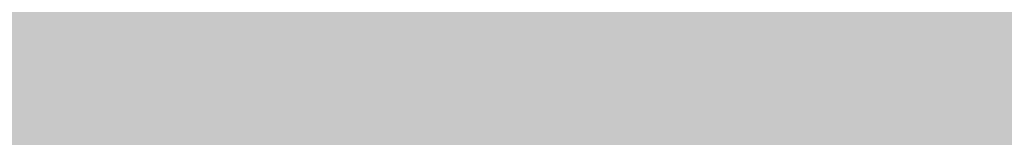
# Model space of a CAD drawing. Units: feet. Extents: x 3168 to 4724, y 827 to 1477.
# Tile 249 of 256: x 3384.3079 to 3384.4267, y 1099.0007 to 1099.0148. Entities that reach past the tile are written whole.
import ezdxf

# ---------------------------------------------------------------- set-up
doc = ezdxf.new("R2010")
doc.units = ezdxf.units.FT
doc.layers.add('A-ELEV', color=7, linetype='Continuous', lineweight=35)
doc.layers.add('A-ELEV-PATT', color=8, linetype='Continuous', lineweight=13)

msp = doc.modelspace()

# ---------------------------------------------------------------- hatches: boundary and pattern name
at = {"layer": 'A-ELEV-PATT'}
h = msp.add_hatch(color=256, dxfattribs=at)
h.dxf.hatch_style = 1
edge = h.paths.add_edge_path()
edge.add_ellipse((3552.90576, 979.22014), major_axis=(36.74492, 0), ratio=0.48484848, start_angle=0, end_angle=360)
edge = h.paths.add_edge_path()
edge.add_ellipse((3559.89164, 929.25228), major_axis=(36.74492, 0), ratio=0.48484848, start_angle=0, end_angle=360)
edge = h.paths.add_edge_path()
edge.add_line((3299.31681, 1198.60608), (3479.91671, 1198.60608))
edge.add_line((3479.91671, 1198.60608), (3479.91671, 1209.86857))
edge.add_spline(control_points=[(3479.91671, 1209.86857), (3464.30116, 1209.86857), (3448.6856, 1209.86857), (3410.94914, 1209.86857), (3388.82823, 1209.86857), (3355.64688, 1209.86857), (3344.58642, 1209.86857), (3327.99574, 1209.86857), (3322.46552, 1209.86857), (3314.17018, 1209.86857), (3311.40507, 1209.86857), (3307.2574, 1209.86857), (3305.87484, 1209.86857), (3303.801, 1209.86857), (3303.10973, 1209.86857), (3302.07281, 1209.86857), (3301.72717, 1209.86857), (3301.20871, 1209.86857), (3301.03589, 1209.86857), (3300.77666, 1209.86857), (3300.69025, 1209.86857), (3300.56064, 1209.86857), (3300.51743, 1209.86857), (3300.45263, 1209.86857), (3300.43102, 1209.86857), (3300.39862, 1209.86857), (3300.38782, 1209.86857), (3300.36622, 1209.86857), (3300.34568, 1209.86857), (3300.34555, 1209.86857), (3300.3455, 1209.86857), (3300.3433, 1209.86857), (3300.34115, 1209.86857), (3300.33791, 1209.86857), (3300.33683, 1209.86857), (3300.33394, 1209.86857), (3300.33213, 1209.86857), (3300.32552, 1209.86858), (3300.32071, 1209.86858), (3300.31092, 1209.86859), (3300.30595, 1209.8686), (3300.29051, 1209.86862), (3300.28005, 1209.86865), (3300.23243, 1209.86878), (3300.1953, 1209.86895), (3299.95107, 1209.87061), (3299.74482, 1209.87433), (3299.43683, 1209.88326), (3299.33439, 1209.88679), (3299.18108, 1209.89292), (3299.13003, 1209.8951), (3298.65222, 1209.9168), (3298.22946, 1209.94572), (3297.60163, 1210.00237), (3297.3934, 1210.02346), (3297.08265, 1210.05831), (3296.97933, 1210.07046), (3296.29295, 1210.15486), (3295.71815, 1210.24336), (3294.86872, 1210.39885), (3294.5877, 1210.45448), (3294.16934, 1210.54335), (3294.03042, 1210.57388), (3291.70715, 1211.1012), (3289.65359, 1211.81344), (3285.77626, 1213.56399), (3283.95141, 1214.60348), (3280.51216, 1216.98008), (3278.89724, 1218.31759), (3276.37991, 1220.82949), (3275.41604, 1221.91774), (3274.03934, 1223.7077), (3273.58104, 1224.34953), (3273.14323, 1225.01632)], knot_values=[39.119033, 39.119033, 39.119033, 39.119033, 39.286353, 39.286353, 39.523379, 39.523379, 39.641892, 39.641892, 39.701148, 39.701148, 39.730777, 39.730777, 39.745591, 39.745591, 39.752998, 39.752998, 39.756701, 39.756701, 39.758553, 39.758553, 39.759479, 39.759479, 39.759942, 39.759942, 39.760173, 39.760173, 39.760289, 39.760289, 39.760405, 39.760405, 39.760463, 39.760463, 39.763389, 39.763389, 39.764851, 39.764851, 39.767304, 39.767304, 39.773825, 39.773825, 39.78057, 39.78057, 39.79477, 39.79477, 39.845194, 39.845194, 40.126715, 40.126715, 40.267476, 40.267476, 40.337856, 40.337856, 40.927023, 40.927023, 41.221606, 41.221606, 41.368898, 41.368898, 42.202622, 42.202622, 42.619485, 42.619485, 42.827916, 42.827916, 46.118323, 46.118323, 49.408731, 49.408731, 52.699139, 52.699139, 54.927489, 54.927489, 56.104228, 56.104228, 56.104228, 56.104228], weights=[1, 1, 1, 1, 1, 1, 1, 1, 1, 1, 1, 1, 1, 1, 1, 1, 1, 1, 1, 1, 1, 1, 1, 1, 1, 1, 1, 1, 1, 1, 1, 1, 1, 1, 1, 1, 1, 1, 1, 1, 1, 1, 1, 1, 1, 1, 1, 1, 1, 1, 1, 1, 1, 1, 1, 1, 1, 1, 1, 1, 1, 1, 1, 1, 1, 1, 1, 1, 1, 1, 1, 1, 1, 1], degree=3, periodic=0)
edge.add_line((3273.14323, 1225.01632), (3273.14323, 1099.01632))
edge.add_line((3273.14323, 1099.01632), (3299.31681, 1099.01632))
edge.add_line((3299.31681, 1099.01632), (3299.31681, 1198.60608))
edge = h.paths.add_edge_path()
edge.add_line((3304.75844, 1324.15806), (3479.91671, 1324.15806))
edge.add_line((3479.91671, 1324.15806), (3479.91671, 1335.71462))
edge.add_line((3479.91671, 1335.71462), (3269.16163, 1335.71462))
edge.add_spline(control_points=[(3269.16163, 1335.71462), (3264.02423, 1335.71462), (3258.36412, 1328.95819), (3259.26431, 1323.90027)], knot_values=[0, 0, 0, 0, 15.412191, 15.412191, 15.412191, 15.412191], degree=3, periodic=0)
edge.add_line((3259.26431, 1323.90027), (3265.51685, 1288.76913))
edge.add_line((3265.51685, 1288.76913), (3275.2651, 1261.54563))
edge.add_line((3275.2651, 1261.54563), (3304.75844, 1261.54563))
edge.add_line((3304.75844, 1261.54563), (3304.75844, 1324.15806))
h = msp.add_hatch(color=256, dxfattribs=at)
h.dxf.hatch_style = 1
h.paths.add_polyline_path([(3384.52525, 1099.01632), (3335.02917, 1099.01632), (3299.31681, 1099.01632), (3273.14323, 1099.01632), (3217.56536, 1099.01632), (3168.06928, 827.11626), (3335.02917, 827.11626)])

# ---------------------------------------------------------------- linework, layer by layer
at = {"layer": 'A-ELEV'}
msp.add_open_spline([(3808.5202, 1099.01632), (3808.5202, 1141.41324), (3808.5202, 1183.81015), (3808.5202, 1226.63532), (3808.5202, 1227.06358), (3808.5202, 1227.49183), (3811.49187, 1248.99467), (3814.46354, 1270.49752), (3817.46523, 1292.21756), (3817.49525, 1292.43476), (3817.52526, 1292.65196), (3817.5728, 1310.10675), (3817.62034, 1327.56153), (3817.66788, 1345.01632), (3817.66788, 1345.45796), (3817.66788, 1345.89961), (3817.66788, 1346.45605), (3817.66788, 1346.57084), (3817.66788, 1346.75289), (3817.66788, 1346.82014), (3817.66788, 1346.93487), (3817.66788, 1346.98234), (3817.66788, 1347.03859), (3817.66788, 1347.04736), (3817.66788, 1347.07366), (3817.66788, 1347.0593), (3817.66788, 1347.06155), (3817.66788, 1347.06267), (3817.66788, 1347.06603), (3817.66787, 1347.06827), (3817.66787, 1347.075), (3817.66787, 1347.07949), (3817.66785, 1347.09294), (3817.66783, 1347.1019), (3817.66777, 1347.12879), (3817.6677, 1347.1467), (3817.66743, 1347.20042), (3817.66716, 1347.23619), (3817.6661, 1347.34338), (3817.66504, 1347.41469), (3817.66081, 1347.62809), (3817.65661, 1347.76971), (3817.63997, 1348.19249), (3817.62351, 1348.47159), (3817.55909, 1349.30007), (3817.49612, 1349.84059), (3817.25543, 1351.42416), (3817.02632, 1352.42879), (3816.30687, 1354.88891), (3815.74375, 1356.26873), (3814.46396, 1358.81921), (3813.74641, 1359.99097), (3812.19584, 1362.17234), (3811.36225, 1363.18212), (3809.58884, 1365.06901), (3808.64882, 1365.94611), (3806.65426, 1367.57962), (3805.5997, 1368.33615), (3803.35289, 1369.72233), (3802.16054, 1370.35239), (3799.60081, 1371.45359), (3798.23269, 1371.92548), (3795.28008, 1372.63462), (3793.69315, 1372.87207), (3791.86944, 1372.92648), (3791.74086, 1372.92922), (3791.35337, 1372.9341), (3791.09271, 1372.9329), (3790.30412, 1372.91507), (3789.76954, 1372.88419), (3789.20919, 1372.83024), (3789.19062, 1372.82842), (3789.13489, 1372.82291), (3789.0977, 1372.81914), (3789.04844, 1372.81401), (3789.0364, 1372.81274), (3789.00026, 1372.80892), (3788.97615, 1372.80633), (3788.9494, 1372.8034), (3788.94679, 1372.80312), (3788.94257, 1372.80266), (3788.94097, 1372.80248), (3788.93857, 1372.80222), (3788.93778, 1372.80213), (3788.93539, 1372.80187), (3788.86753, 1372.7944), (3788.75687, 1372.78223), (3788.70153, 1372.77614), (3788.53553, 1372.75788), (3788.42486, 1372.74571), (3788.09286, 1372.70918), (3787.87152, 1372.68484), (3787.20751, 1372.61179), (3786.76483, 1372.5631), (3785.43681, 1372.41701), (3784.55147, 1372.31962), (3781.89542, 1372.02744), (3780.12473, 1371.83266), (3774.81265, 1371.24831), (3771.27126, 1370.85874), (3760.64709, 1369.69004), (3753.56431, 1368.9109), (3732.31597, 1366.5735), (3718.15042, 1365.01523), (3694.00676, 1362.35933), (3684.02866, 1361.26169), (3674.05056, 1360.16406), (3664.60066, 1360.16406), (3655.15077, 1360.16406), (3626.80108, 1360.16406), (3607.90129, 1360.16406), (3551.20192, 1360.16406), (3513.40234, 1360.16406), (3467.72518, 1360.16406), (3459.8476, 1360.16406), (3436.21487, 1360.16406), (3420.45972, 1360.16406), (3373.19425, 1360.16406), (3341.68395, 1360.16406), (3302.84816, 1360.16406), (3295.52269, 1360.16406), (3286.03829, 1360.16406), (3283.87937, 1360.16406), (3277.40261, 1360.16406), (3273.08477, 1360.16406), (3267.73285, 1360.16406), (3266.69877, 1360.16406), (3263.59652, 1360.16406), (3261.52835, 1360.16406), (3259.23694, 1360.16406), (3259.0137, 1360.16406), (3258.34396, 1360.16406), (3257.89747, 1360.16406), (3257.431, 1360.16406), (3257.41102, 1360.16406), (3257.37057, 1360.16406), (3257.37547, 1360.16406), (3257.3746, 1360.16406), (3257.37394, 1360.16406), (3257.37196, 1360.16406), (3257.37064, 1360.16406), (3257.36667, 1360.16406), (3257.36403, 1360.16406), (3257.35611, 1360.16405), (3257.35083, 1360.16405), (3257.33499, 1360.16402), (3257.32443, 1360.164), (3257.29277, 1360.1639), (3257.27168, 1360.1638), (3257.20844, 1360.1634), (3257.16634, 1360.163), (3257.04021, 1360.16139), (3256.95635, 1360.15978), (3256.7055, 1360.15339), (3256.53924, 1360.14704), (3256.04357, 1360.12192), (3255.7173, 1360.0971), (3254.75245, 1360.00048), (3254.12797, 1359.90651), (3252.18007, 1359.52533), (3250.94157, 1359.14399), (3248.67018, 1358.24329), (3247.63574, 1357.72383), (3245.73263, 1356.60347), (3244.86339, 1356.00206), (3243.25311, 1354.74287), (3242.51197, 1354.08473), (3240.75105, 1352.34478), (3239.80096, 1351.22957), (3238.08777, 1348.87244), (3237.32469, 1347.63036), (3235.98251, 1344.97163), (3235.40221, 1343.55491), (3234.59108, 1340.81546), (3234.31088, 1339.54355), (3233.97649, 1336.80256), (3233.92211, 1335.33088), (3234.14892, 1332.59127), (3234.34953, 1331.3672), (3234.71989, 1329.99937), (3234.75242, 1329.88336), (3234.85362, 1329.5348), (3234.92589, 1329.30168), (3235.02484, 1329.00255), (3235.04692, 1328.93693), (3235.07764, 1328.84724), (3235.08592, 1328.8232), (3235.11094, 1328.75106), (3235.12783, 1328.70296), (3235.14799, 1328.64624), (3235.15106, 1328.63763), (3235.1561, 1328.62353), (3235.15806, 1328.61803), (3235.16021, 1328.61203), (3235.16561, 1328.59694), (3235.1801, 1328.55649), (3235.19026, 1328.5281), (3235.22076, 1328.44295), (3235.24108, 1328.38618), (3235.30207, 1328.21587), (3235.34273, 1328.10232), (3235.4647, 1327.7617), (3235.54601, 1327.53462), (3235.78995, 1326.85338), (3235.95258, 1326.39922), (3236.44046, 1325.03674), (3236.76571, 1324.12841), (3237.74148, 1321.40345), (3238.39198, 1319.5868), (3240.34351, 1314.13687), (3241.64452, 1310.50358), (3245.54757, 1299.60371), (3248.14961, 1292.33713), (3255.95571, 1270.53739), (3261.15977, 1256.00423), (3267.38762, 1238.612), (3268.4114, 1235.75294), (3269.51038, 1232.68386), (3269.58558, 1232.47385), (3269.70661, 1232.13585), (3269.75244, 1232.00786), (3269.82733, 1231.79873), (3269.85638, 1231.7176), (3269.90632, 1231.57812), (3269.92721, 1231.51978), (3269.97247, 1231.39341), (3269.99683, 1231.32537), (3270.0265, 1231.24251), (3270.03181, 1231.22768), (3270.04028, 1231.20402), (3270.03922, 1231.20698), (3270.03936, 1231.2066), (3270.03943, 1231.20641), (3270.03963, 1231.20585), (3270.03977, 1231.20547), (3270.04017, 1231.20433), (3270.04044, 1231.20358), (3270.04125, 1231.20131), (3270.0418, 1231.1998), (3270.04342, 1231.19527), (3270.0445, 1231.19225), (3270.04776, 1231.18318), (3270.04993, 1231.17714), (3270.05644, 1231.15903), (3270.06079, 1231.14696), (3270.07387, 1231.11076), (3270.08261, 1231.08666), (3270.10894, 1231.01441), (3270.1266, 1230.96635), (3270.17993, 1230.82246), (3270.21595, 1230.72692), (3270.32532, 1230.44151), (3270.40003, 1230.25281), (3270.62925, 1229.69144), (3270.78888, 1229.3235), (3271.28649, 1228.23832), (3271.6431, 1227.53975), (3272.77586, 1225.51528), (3273.61417, 1224.2605), (3275.41604, 1221.91774), (3276.37991, 1220.82949), (3278.89724, 1218.31759), (3280.51216, 1216.98008), (3283.95141, 1214.60348), (3285.77626, 1213.56399), (3289.65359, 1211.81344), (3291.70715, 1211.1012), (3294.03042, 1210.57388), (3294.16934, 1210.54335), (3294.5877, 1210.45448), (3294.86872, 1210.39885), (3295.71815, 1210.24336), (3296.29295, 1210.15486), (3296.97933, 1210.07046), (3297.08265, 1210.05831), (3297.3934, 1210.02346), (3297.60163, 1210.00237), (3298.22946, 1209.94572), (3298.65222, 1209.9168), (3299.13003, 1209.8951), (3299.18108, 1209.89292), (3299.33439, 1209.88679), (3299.43683, 1209.88326), (3299.74482, 1209.87433), (3299.95107, 1209.87061), (3300.1953, 1209.86895), (3300.23243, 1209.86878), (3300.28005, 1209.86865), (3300.29051, 1209.86862), (3300.30595, 1209.8686), (3300.31092, 1209.86859), (3300.32071, 1209.86858), (3300.32552, 1209.86858), (3300.33213, 1209.86857), (3300.33394, 1209.86857), (3300.33683, 1209.86857), (3300.33791, 1209.86857), (3300.34115, 1209.86857), (3300.3433, 1209.86857), (3300.3455, 1209.86857), (3300.34555, 1209.86857), (3300.34568, 1209.86857), (3300.36622, 1209.86857), (3300.38782, 1209.86857), (3300.39862, 1209.86857), (3300.43102, 1209.86857), (3300.45263, 1209.86857), (3300.51743, 1209.86857), (3300.56064, 1209.86857), (3300.69025, 1209.86857), (3300.77666, 1209.86857), (3301.03589, 1209.86857), (3301.20871, 1209.86857), (3301.72717, 1209.86857), (3302.07281, 1209.86857), (3303.10973, 1209.86857), (3303.801, 1209.86857), (3305.87484, 1209.86857), (3307.2574, 1209.86857), (3311.40507, 1209.86857), (3314.17018, 1209.86857), (3322.46552, 1209.86857), (3327.99574, 1209.86857), (3344.58642, 1209.86857), (3355.64688, 1209.86857), (3388.82823, 1209.86857), (3410.94914, 1209.86857), (3477.31185, 1209.86857), (3521.55366, 1209.86857), (3566.83618, 1209.86857), (3567.87689, 1209.86857), (3570.99902, 1209.86857), (3573.08043, 1209.86857), (3575.7814, 1209.86857), (3576.40094, 1209.86857), (3577.29582, 1209.86857), (3577.57115, 1209.86857), (3578.39715, 1209.86857), (3578.94781, 1209.86857), (3579.75649, 1209.86857), (3580.01451, 1209.86857), (3580.34274, 1209.86857), (3580.32686, 1209.86857), (3580.32717, 1209.86857), (3580.32732, 1209.86857), (3580.32778, 1209.86857), (3580.32809, 1209.86857), (3580.329, 1209.86857), (3580.32961, 1209.86857), (3580.33145, 1209.86857), (3580.33267, 1209.86857), (3580.33633, 1209.86857), (3580.33878, 1209.86857), (3580.34611, 1209.86856), (3580.35099, 1209.86856), (3580.36566, 1209.86854), (3580.37544, 1209.86852), (3580.4048, 1209.86845), (3580.42439, 1209.86838), (3580.48318, 1209.86808), (3580.52244, 1209.86779), (3580.64036, 1209.86662), (3580.71919, 1209.86545), (3580.95632, 1209.86077), (3581.11522, 1209.85607), (3581.59416, 1209.83723), (3581.91642, 1209.81833), (3582.88995, 1209.74243), (3583.54799, 1209.66617), (3585.53183, 1209.36062), (3586.86722, 1209.05389), (3589.47155, 1208.25247), (3590.74024, 1207.75785), (3591.99545, 1207.1588), (3592.05781, 1207.12874), (3592.24424, 1207.03795), (3592.36768, 1206.97663), (3592.73528, 1206.79036), (3592.97675, 1206.6631), (3593.24454, 1206.51644), (3593.27473, 1206.49982), (3593.36512, 1206.44984), (3593.42511, 1206.41633), (3593.60431, 1206.31529), (3593.72273, 1206.24721), (3593.85721, 1206.1684), (3593.87436, 1206.15832), (3593.92574, 1206.12804), (3593.9599, 1206.1078), (3594.06209, 1206.0469), (3594.12983, 1206.00607), (3594.20844, 1205.95817), (3594.21968, 1205.9513), (3594.25339, 1205.93069), (3594.27582, 1205.91692), (3594.34297, 1205.87554), (3594.38756, 1205.84785), (3594.43362, 1205.81905), (3594.43526, 1205.81802), (3594.44017, 1205.81495), (3594.44345, 1205.81289), (3594.44712, 1205.81059), (3594.44752, 1205.81035), (3594.44869, 1205.80961), (3594.44948, 1205.80912), (3594.45037, 1205.80856), (3594.45047, 1205.8085), (3594.4506, 1205.80842), (3594.4674, 1205.79789), (3594.49327, 1205.78167), (3594.5062, 1205.77357), (3594.54501, 1205.74925), (3594.57088, 1205.73303), (3594.64849, 1205.6844), (3594.70023, 1205.65197), (3594.85544, 1205.55469), (3594.95892, 1205.48984), (3595.26936, 1205.29528), (3595.47631, 1205.16558), (3596.09719, 1204.77646), (3596.5111, 1204.51705), (3597.75284, 1203.73883), (3598.58067, 1203.22001), (3601.06415, 1201.66355), (3602.71981, 1200.62591), (3607.68677, 1197.513), (3610.99809, 1195.43773), (3620.93202, 1189.2119), (3627.55464, 1185.06135), (3647.42251, 1172.60971), (3660.66775, 1164.30861), (3700.40348, 1139.40531), (3726.89397, 1122.80312), (3757.20572, 1103.80605), (3761.02697, 1101.41118), (3764.84822, 1099.01632), (3745.32827, 1099.01632), (3725.80832, 1099.01632), (3706.28837, 1099.01632), (3706.28837, 1108.45324), (3706.28837, 1117.89016), (3706.28837, 1127.32708), (3710.75075, 1127.32708), (3715.21314, 1127.32708), (3719.67553, 1127.32708)], degree=3, knots=[0, 0, 0, 0, 0.982037, 0.982037, 0.991957, 0.991957, 0.991957, 1.966522, 1.966522, 1.976367, 1.976367, 1.976367, 2.976367, 2.976367, 2.976367, 3.00169, 3.00169, 3.008272, 3.008272, 3.012129, 3.012129, 3.014851, 3.014851, 3.015353, 3.015353, 3.016359, 3.016359, 3.017365, 3.017365, 3.019376, 3.019376, 3.023398, 3.023398, 3.031442, 3.031442, 3.047531, 3.047531, 3.079708, 3.079708, 3.144063, 3.144063, 3.272772, 3.272772, 3.53019, 3.53019, 4.045026, 4.045026, 5.074698, 5.074698, 6.700878, 6.700878, 8.327058, 8.327058, 9.953238, 9.953238, 11.579418, 11.579418, 13.205598, 13.205598, 14.831778, 14.831778, 16.457958, 16.457958, 18.084138, 18.084138, 18.206872, 18.206872, 18.45234, 18.45234, 18.943275, 18.943275, 18.960093, 18.960093, 18.993729, 18.993729, 19.00461, 19.00461, 19.026374, 19.026374, 19.028737, 19.028737, 19.03018, 19.03018, 19.030897, 19.030897, 19.032332, 19.032332, 19.033766, 19.033766, 19.036636, 19.036636, 19.042374, 19.042374, 19.053851, 19.053851, 19.076805, 19.076805, 19.122714, 19.122714, 19.21453, 19.21453, 19.398163, 19.398163, 19.765429, 19.765429, 20.024128, 20.024128, 20.024128, 20.092031, 20.092031, 20.227836, 20.227836, 20.499446, 20.499446, 20.556051, 20.556051, 20.66926, 20.66926, 20.895678, 20.895678, 20.948316, 20.948316, 20.963829, 20.963829, 20.994855, 20.994855, 21.002285, 21.002285, 21.017146, 21.017146, 21.01875, 21.01875, 21.021959, 21.021959, 21.022102, 21.022102, 21.022249, 21.022249, 21.022708, 21.022708, 21.023627, 21.023627, 21.025464, 21.025464, 21.029138, 21.029138, 21.036486, 21.036486, 21.051183, 21.051183, 21.080575, 21.080575, 21.139361, 21.139361, 21.256932, 21.256932, 21.492073, 21.492073, 21.962356, 21.962356, 23.01002, 23.01002, 24.057684, 24.057684, 25.105348, 25.105348, 26.153011, 26.153011, 27.776787, 27.776787, 29.400562, 29.400562, 31.024337, 31.024337, 32.278801, 32.278801, 33.533265, 33.533265, 34.467568, 34.467568, 34.553971, 34.553971, 34.726776, 34.726776, 34.775309, 34.775309, 34.793079, 34.793079, 34.82862, 34.82862, 34.834979, 34.834979, 34.839039, 34.839039, 34.839411, 34.839411, 34.840285, 34.840285, 34.842034, 34.842034, 34.845531, 34.845531, 34.852525, 34.852525, 34.866512, 34.866512, 34.894488, 34.894488, 34.950439, 34.950439, 35.062342, 35.062342, 35.286147, 35.286147, 35.733758, 35.733758, 35.821815, 35.821815, 35.828283, 35.828283, 35.832225, 35.832225, 35.834724, 35.834724, 35.836521, 35.836521, 35.838617, 35.838617, 35.839073, 35.839073, 35.839345, 35.839345, 35.839617, 35.839617, 35.840161, 35.840161, 35.841249, 35.841249, 35.843425, 35.843425, 35.847778, 35.847778, 35.856482, 35.856482, 35.873891, 35.873891, 35.908709, 35.908709, 35.978345, 35.978345, 36.117617, 36.117617, 36.396161, 36.396161, 36.953248, 36.953248, 38.067423, 38.067423, 40.295772, 40.295772, 42.524122, 42.524122, 45.81453, 45.81453, 49.104937, 49.104937, 52.395345, 52.395345, 52.603776, 52.603776, 53.020639, 53.020639, 53.854363, 53.854363, 54.001655, 54.001655, 54.296238, 54.296238, 54.885405, 54.885405, 54.955785, 54.955785, 55.096546, 55.096546, 55.378067, 55.378067, 55.42849, 55.42849, 55.442691, 55.442691, 55.449436, 55.449436, 55.455957, 55.455957, 55.458409, 55.458409, 55.459872, 55.459872, 55.462798, 55.462798, 55.462856, 55.462856, 55.462972, 55.462972, 55.463088, 55.463088, 55.463319, 55.463319, 55.463782, 55.463782, 55.464708, 55.464708, 55.46656, 55.46656, 55.470263, 55.470263, 55.47767, 55.47767, 55.492484, 55.492484, 55.522112, 55.522112, 55.581369, 55.581369, 55.699882, 55.699882, 55.936907, 55.936907, 56.410959, 56.410959, 56.42211, 56.42211, 56.444413, 56.444413, 56.451051, 56.451051, 56.454001, 56.454001, 56.459901, 56.459901, 56.462666, 56.462666, 56.463418, 56.463418, 56.464171, 56.464171, 56.465675, 56.465675, 56.468684, 56.468684, 56.474702, 56.474702, 56.486738, 56.486738, 56.51081, 56.51081, 56.558955, 56.558955, 56.655243, 56.655243, 56.847821, 56.847821, 57.232975, 57.232975, 58.003284, 58.003284, 59.543901, 59.543901, 62.625137, 62.625137, 68.787607, 68.787607, 74.950078, 74.950078, 75.27336, 75.27336, 75.919923, 75.919923, 77.213051, 77.213051, 77.377769, 77.377769, 77.707206, 77.707206, 78.366079, 78.366079, 78.462532, 78.462532, 78.655436, 78.655436, 79.041245, 79.041245, 79.105735, 79.105735, 79.234714, 79.234714, 79.492672, 79.492672, 79.502197, 79.502197, 79.521249, 79.521249, 79.523534, 79.523534, 79.528103, 79.528103, 79.528682, 79.528682, 79.528885, 79.528885, 79.529089, 79.529089, 79.529495, 79.529495, 79.530308, 79.530308, 79.531935, 79.531935, 79.535187, 79.535187, 79.541693, 79.541693, 79.554704, 79.554704, 79.580725, 79.580725, 79.632769, 79.632769, 79.736856, 79.736856, 79.94503, 79.94503, 80.361377, 80.361377, 80.421435, 80.421435, 80.421435, 81.421435, 81.421435, 81.421435, 82.421435, 82.421435, 82.421435, 83.421435, 83.421435, 83.421435, 83.421435], dxfattribs=at)

doc.saveas('drawing.dxf')
